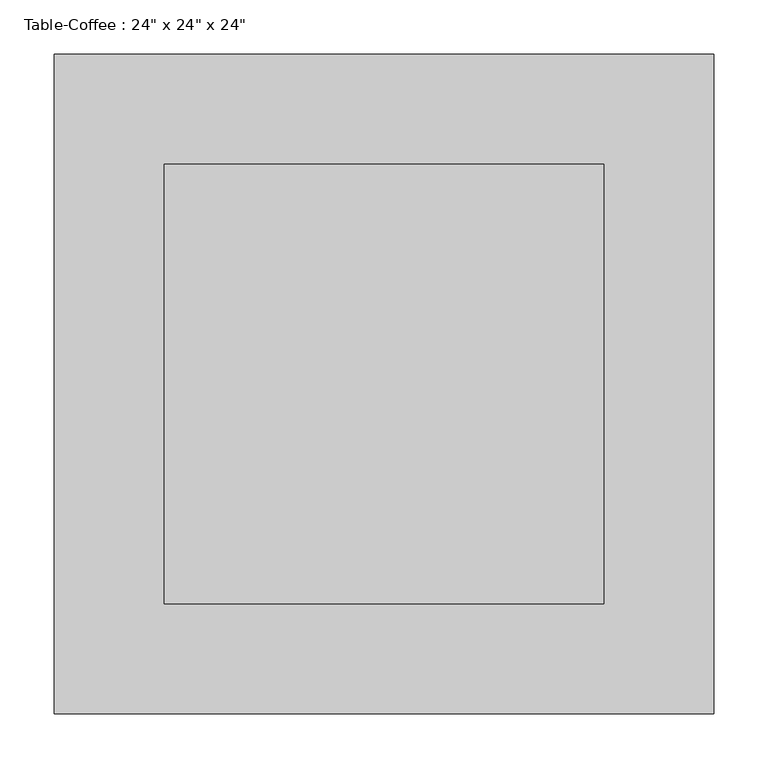
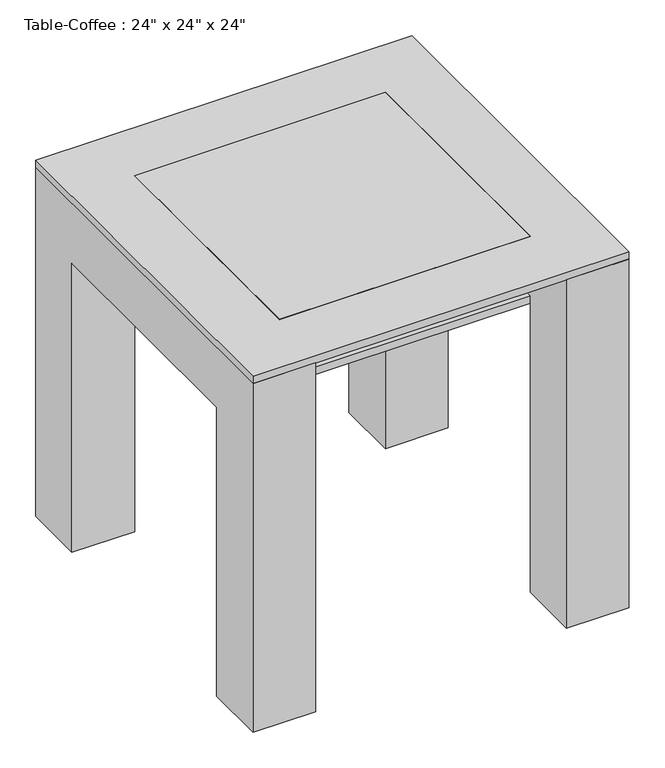
"""IFC4 building model written with IfcOpenShell, lengths in millimetres: furniture geometry."""

from ifc_helpers import new_model, si_unit, frame, origin, place, context, project, spatial, polyline, outline, extrude, source, transform, mapped, element, save


def furniture_b5c51a22(model_context):
    return source(origin(), model_context, "Body", "SweptSolid", [
        extrude(outline(polyline([(221.4657667, 298.4110778), (221.4657667, -107.9889222), (-184.9342333, -107.9889222), (-184.9342333, 298.4110778), (221.4657667, 298.4110778)])), frame((0.0, 0.0, 495.3), z_axis=(0.0, 0.0, 1.0), x_axis=(1.0, 0.0, 0.0)), (0.0, 0.0, 1.0), 12.7),
        extrude(outline(polyline([(400.0110778, 0.0), (298.4110778, 0.0), (298.4110778, 495.3), (-107.9889222, 495.3), (-107.9889222, 0.0), (-209.5889222, 0.0), (-209.5889222, 596.9), (400.0110778, 596.9), (400.0110778, 0.0)])), frame((221.4657667, 0.0, 0.0), z_axis=(1.0, 0.0, 0.0), x_axis=(0.0, 1.0, 0.0)), (0.0, 0.0, 1.0), 101.6),
        extrude(outline(polyline([(400.0110778, 596.9), (400.0110778, 0.0), (298.4110778, 0.0), (298.4110778, 495.3), (-107.9889222, 495.3), (-107.9889222, 0.0), (-209.5889222, 0.0), (-209.5889222, 596.9), (400.0110778, 596.9)])), frame((-286.5342333, 0.0, 0.0), z_axis=(1.0, 0.0, 0.0), x_axis=(0.0, 1.0, 0.0)), (0.0, 0.0, 1.0), 101.6),
        extrude(outline(polyline([(221.4657667, 298.4110778), (221.4657667, -107.9889222), (-184.9342333, -107.9889222), (-184.9342333, 298.4110778), (221.4657667, 298.4110778)])), frame((0.0, 0.0, 596.9), z_axis=(0.0, 0.0, 1.0), x_axis=(1.0, 0.0, 0.0)), (0.0, 0.0, 1.0), 12.7),
        extrude(outline(polyline([(323.0657667, 400.0110778), (323.0657667, -209.5889222), (-286.5342333, -209.5889222), (-286.5342333, 400.0110778), (323.0657667, 400.0110778)]), holes=[polyline([(221.4657667, 298.4110778), (-184.9342333, 298.4110778), (-184.9342333, -107.9889222), (221.4657667, -107.9889222), (221.4657667, 298.4110778)])]), frame((0.0, 0.0, 596.9), z_axis=(0.0, 0.0, 1.0), x_axis=(1.0, 0.0, 0.0)), (0.0, 0.0, 1.0), 12.7),
    ])


if __name__ == "__main__":
    model = new_model("IFC4")
    model_context = context("Model", 3, world=origin())
    ifc_project = project(units=[si_unit("LENGTHUNIT", "METRE", prefix="MILLI")], contexts=[model_context])
    site = spatial("IfcSite", under=ifc_project)
    building = spatial("IfcBuilding", under=site)
    placement = place(None, origin())
    furniture_shape = furniture_b5c51a22(model_context)
    element("IfcFurniture", 1, ObjectType="Table-Coffee : 24\" x 24\" x 24\"", at=placement, inside=building, context=model_context, shape_type="MappedRepresentation", body=[
        mapped(furniture_shape, transform((0.0, 0.0, 0.0), x_axis=(1.0, 0.0, 0.0), y_axis=(0.0, 1.0, 0.0), z_axis=(0.0, 0.0, 1.0))),
    ])
    save(model, "model.ifc")

# Revit data of these elements
# Type "Table-Coffee : 24\" x 24\" x 24\""
#   Assembly Code = "E2020200"
#   Height = 2' - 0"
#   Length = 2' - 0"
#   Width = 2' - 0"
#   Top Material = none
#   Frame Material = none
#   Default Elevation = 0
# Element 1 (IfcFurniture, "Table-Coffee : 24\" x 24\" x 24\"")
#   Materials on its faces: "Glass - Clear, Grey"
# Materials
#   "Glass - Clear, Grey": class "Glass", colour RGB 252 255 255, transparency 0.64
